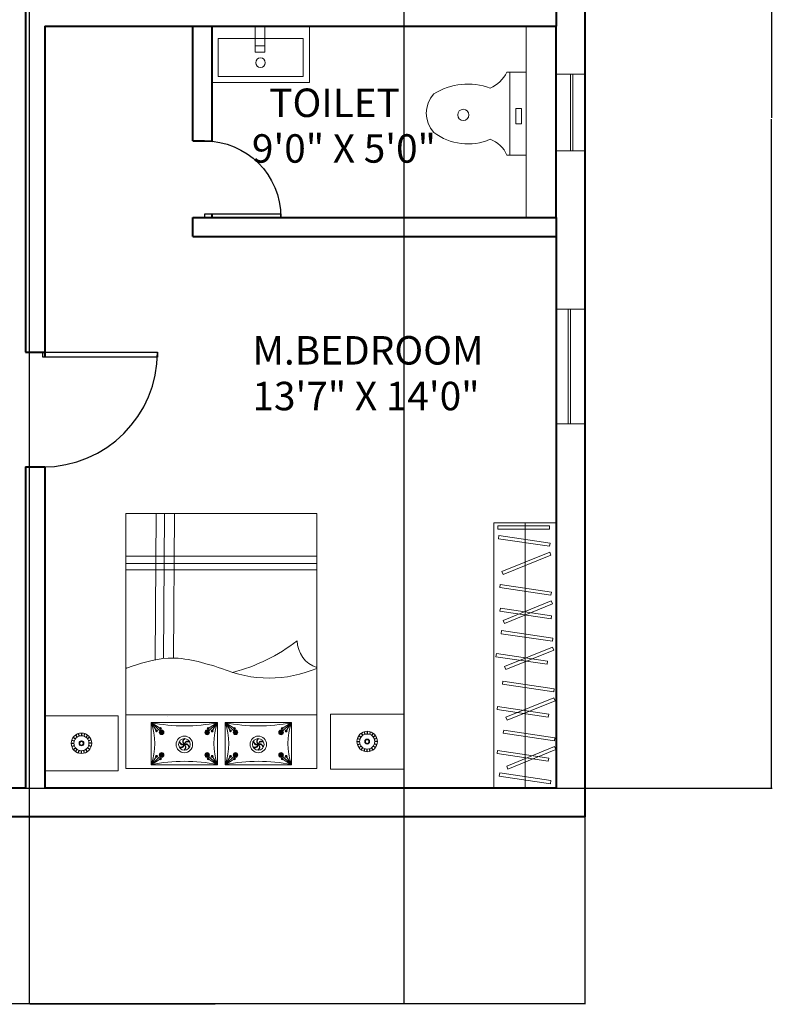
# Model space of a CAD drawing. Units: inches. Extents: x -46 to 1145, y -527 to 760.
# Tile 19 of 57: x 909 to 1145, y -527 to -218. Entities that reach past the tile are written whole.
import ezdxf

# ---------------------------------------------------------------- set-up
doc = ezdxf.new("R2010")
doc.units = ezdxf.units.IN
doc.header["$MEASUREMENT"] = 0
for name, color, linetype, lineweight in [('A-ANNO-DIMS', 2, 'Continuous', 18), ('A-AREA-IDEN', 1, 'Continuous', 18), ('A-FLOR-CASE', 32, 'Continuous', 18), ('A-FLOR-FIXT', 9, 'Continuous', 18), ('A-FURN', 2, 'Continuous', 13), ('C-SITE', 7, 'Continuous', 30), ('DOORS', 3, 'Continuous', 25), ('WALLS', 4, 'Continuous', 40), ('WINDOWS', 240, 'Continuous', 20)]:
    doc.layers.add(name, color=color, linetype=linetype, lineweight=lineweight)
doc.layers.add('FURNTIURE', color=2, linetype='Continuous')
doc.layers.add('LT', color=9, linetype='Continuous')
doc.styles.get("Standard").update_dxf_attribs({"font": 'arial.ttf'})
doc.dimstyles.get("Standard").update_dxf_attribs({"dimtxt": 0.18, "dimasz": 0.18, "dimexe": 0.18, "dimexo": 0.0625, "dimgap": 0.09, "dimtad": 0, "dimtih": 1, "dimtoh": 1, "dimdec": 0, "dimzin": 0, "dimdsep": 46, "dimlunit": 3, "dimtxsty": 'Standard', "dimcen": 0.09, "dimadec": 0, "dimazin": 0, "dimtfac": 1, "dimtdec": 0, "dimtofl": 0, "dimtmove": 0, "dimatfit": 3, "dimfxl": 1, "dimtolj": 1, "dimtzin": 0, "dimarcsym": 0})

# ---------------------------------------------------------------- blocks, each defined once
blk = doc.blocks.new('*U2')
for p, q in [((0, 0), (0, -6)), ((40, 0), (40, -6))]:
    blk.add_line(p, q)
blk.add_lwpolyline([(0, 0), (0, 40), (1.75, 40), (1.75, 0)], close=True)
blk.add_arc((0, 0), 40, 0, 90)
blk = doc.blocks.new('*U89')
at = {"layer": 'FURNTIURE'}
blk.add_line((0, 0.42), (0, -0.42), dxfattribs=at)
blk = doc.blocks.new('*U90')
at = {"layer": 'FURNTIURE', "transparency": 16777216}
for p, rotation in [((589.5, 506.39), 54), ((590.11, 507), 36), ((590.89, 507.4), 17.99999999999997), ((592.61, 507.4), 341.9999999999999), ((593.39, 507), 324), ((594.01, 506.39), 306), ((588.97, 504.75), 90), ((589.1, 505.61), 72), ((589.1, 503.89), 108), ((589.5, 503.11), 126), ((594.01, 503.11), 234), ((594.4, 505.61), 288), ((594.4, 503.89), 252), ((594.54, 504.75), 270), ((590.11, 502.49), 144), ((590.89, 502.1), 162), ((591.75, 501.96), 180), ((592.61, 502.1), 197.9999999999999), ((593.39, 502.49), 216)]:
    blk.add_blockref('*U89', p, dxfattribs=dict(at, rotation=rotation))
blk.add_blockref('*U89', (591.75, 507.53), dxfattribs=at)
blk = doc.blocks.new('*U87')
at = {"layer": 'FURNTIURE'}
blk.add_line((0, 0.1), (0, -0.1), dxfattribs=at)
blk = doc.blocks.new('*U88')
at = {"layer": 'FURNTIURE', "transparency": 16777216}
for p, rotation in [((141.23, 121.04), 90), ((141.27, 121.25), 72), ((141.27, 120.83), 108), ((141.36, 121.43), 54), ((141.36, 120.65), 126), ((141.51, 121.58), 35.99999999999999), ((141.51, 120.5), 144), ((141.7, 121.67), 17.99999999999998), ((141.7, 120.4), 162), ((141.9, 120.37), 180), ((142.11, 121.67), 342), ((142.11, 120.4), 198), ((142.3, 121.58), 324), ((142.3, 120.5), 216), ((142.44, 121.43), 306), ((142.44, 120.65), 234), ((142.54, 121.25), 288), ((142.54, 120.83), 252), ((142.57, 121.04), 270)]:
    blk.add_blockref('*U87', p, dxfattribs=dict(at, rotation=rotation))
blk.add_blockref('*U87', (141.9, 121.71), dxfattribs=at)
blk = doc.blocks.new('NIGHTSTAND')
blk.add_lwpolyline([(23.06, 0), (0, 0), (0, 17.28), (23.06, 17.28)], close=True)
for radius in [3.21, 2.36, 0.77, 0.567]:
    blk.add_circle((11.53, 8.64), radius)
for name, p in [('*U90', (-580.22, -496.1)), ('*U88', (-130.37, -112.4))]:
    blk.add_blockref(name, p)
blk = doc.blocks.new('WARDROBE')
blk.add_line((9.78, 0), (9.78, 83.25))
for points in [[(19.56, 0), (0, 0), (0, 83.25), (19.56, 83.25)], [(17.74, 78.49), (1.66, 80.88), (1.8, 81.87), (17.88, 79.48)], [(15.55, 76.35), (0.49, 70.23), (0.11, 71.16), (15.17, 77.28)], [(18.43, 71.4), (2.35, 73.79), (2.5, 74.78), (18.58, 72.39)], [(16.47, 65.03), (0.39, 67.42), (0.54, 68.41), (16.62, 66.02)], [(15.79, 61), (0.73, 54.88), (0.35, 55.81), (15.41, 61.93)], [(18.43, 57.62), (2.35, 60.01), (2.5, 61), (18.58, 58.61)], [(16.71, 49.68), (0.63, 52.07), (0.78, 53.06), (16.86, 50.67)], [(16.22, 45.12), (1.16, 39), (0.78, 39.93), (15.84, 46.05)], [(18.77, 41.02), (2.69, 43.41), (2.84, 44.4), (18.92, 42.01)], [(17.14, 33.8), (1.06, 36.19), (1.21, 37.19), (17.29, 34.8)], [(16.65, 30.67), (1.59, 24.55), (1.21, 25.48), (16.27, 31.6)], [(17.52, 26.78), (1.44, 29.17), (1.59, 30.16), (17.67, 27.77)], [(17.57, 19.35), (1.49, 21.74), (1.64, 22.73), (17.72, 20.34)], [(17.08, 15.35), (2.02, 9.23), (1.64, 10.16), (16.7, 16.28)], [(18, 4.03), (1.92, 6.42), (2.07, 7.41), (18.15, 5.03)], [(18.32, 0.98), (2.07, 0.98), (2.07, 1.98), (18.32, 1.98)]]:
    blk.add_lwpolyline(points, close=True)
blk = doc.blocks.new('LAVATORY-RECT')
blk.add_line((14.01, 6.17), (17.08, 6.17))
for points in [[(30.61, 0), (0, 0), (0, 17.7), (30.61, 17.7)], [(28.7, 3.94), (1.97, 3.94), (1.97, 15.81), (28.7, 15.81)], [(17.08, 0), (14.01, 0), (14.01, 8.17), (17.08, 8.17)]]:
    blk.add_lwpolyline(points, close=True)
blk.add_circle((15.39, 11.51), 1.51)
blk = doc.blocks.new('WATER-CLOSET')
for p, q in [((0, 0), (0, 26.01)), ((0, 26.01), (6.13, 26.01)), ((5.22, 21.04), (5.22, 26.01)), ((5.22, 26.01), (5.22, 0)), ((0, 0), (6.13, 0))]:
    blk.add_line(p, q)
blk.add_lwpolyline([(1.51, 11.4), (1.51, 16.16), (3.34, 16.16), (3.34, 11.4)], close=True)
blk.add_circle((19.79, 13.37), 1.75)
for centre, radius, start, end in [((14.15, 29.2), 8.64, 201.6782, 251.0259), ((18.35, 4.96), 17.54, 52.4616, 113.5359), ((22.52, 12.84), 8.87, 317.2682, 42.7318), ((18.33, 23.71), 20, 249.5645, 302.3709), ((15.4, -4.5), 10.31, 113.1704, 154.0947)]:
    blk.add_arc(centre, radius, start, end)
blk = doc.blocks.new('WINDOW-36IN')
for p, q in [((0, 4.5), (0, 9)), ((0, 9), (0, 0)), ((36, 9), (36, 0)), ((0, 5.23), (36, 5.23)), ((0, 4.5), (36, 4.5))]:
    blk.add_line(p, q)
blk = doc.blocks.new('WINDOW-24IN')
for p, q in [((0, 4.5), (0, 9)), ((0, 9), (0, 0)), ((24, 9), (24, 0)), ((0, 5.23), (24, 5.23)), ((0, 4.5), (24, 4.5))]:
    blk.add_line(p, q)
blk = doc.blocks.new('*U58')
at = {"layer": 'LT'}
blk.add_line((0, 0.28), (0, -0.28), dxfattribs=at)
for centre, start, end in [((0.73, 0), 159.0676, 200.9324), ((-0.73, 0), 339.0676, 20.9324)]:
    blk.add_arc(centre, 0.786, start, end, dxfattribs=at)
blk = doc.blocks.new('*U59')
at = {"layer": 'LT', "transparency": 16777216}
for p, rotation in [((609.66, 443.79), 80.00000000000001), ((609.69, 443.6), 120), ((609.76, 443.96), 40.00000000000002), ((609.84, 443.48), 160), ((610.03, 443.48), 200), ((610.12, 443.96), 320), ((610.18, 443.6), 240), ((610.21, 443.79), 280)]:
    blk.add_blockref('*U58', p, dxfattribs=dict(at, rotation=rotation))
blk.add_blockref('*U58', (609.94, 444.03), dxfattribs=at)
blk = doc.blocks.new('*U60')
at = {"layer": 'LT'}
blk.add_line((0, 0.12), (0, -0.12), dxfattribs=at)
for centre, start, end in [((0.31, 0), 159.0676, 200.9324), ((-0.31, 0), 339.0676, 20.9324)]:
    blk.add_arc(centre, 0.335, start, end, dxfattribs=at)
blk = doc.blocks.new('*U61')
at = {"layer": 'LT', "transparency": 16777216}
for p, rotation in [((259.5, 188.9), 80.00000000000001), ((259.51, 188.82), 120), ((259.54, 188.97), 40), ((259.57, 188.76), 160), ((259.65, 188.76), 200), ((259.69, 188.97), 320), ((259.72, 188.82), 240), ((259.73, 188.9), 280)]:
    blk.add_blockref('*U60', p, dxfattribs=dict(at, rotation=rotation))
blk.add_blockref('*U60', (259.61, 189), dxfattribs=at)
blk = doc.blocks.new('*U62')
at = {"layer": 'LT'}
blk.add_line((0, 0.12), (0, -0.12), dxfattribs=at)
for centre, start, end in [((0.31, 0), 159.0676, 200.9324), ((-0.31, 0), 339.0676, 20.9324)]:
    blk.add_arc(centre, 0.335, start, end, dxfattribs=at)
blk = doc.blocks.new('*U63')
at = {"layer": 'LT', "transparency": 16777216}
for p, rotation in [((259.5, 188.9), 80.00000000000001), ((259.51, 188.82), 120), ((259.54, 188.97), 40), ((259.57, 188.76), 160), ((259.65, 188.76), 200), ((259.69, 188.97), 320), ((259.72, 188.82), 240), ((259.73, 188.9), 280)]:
    blk.add_blockref('*U62', p, dxfattribs=dict(at, rotation=rotation))
blk.add_blockref('*U62', (259.61, 189), dxfattribs=at)
blk = doc.blocks.new('*U64')
at = {"layer": 'LT'}
blk.add_line((0, 0.28), (0, -0.28), dxfattribs=at)
for centre, start, end in [((0.73, 0), 159.0676, 200.9324), ((-0.73, 0), 339.0676, 20.9324)]:
    blk.add_arc(centre, 0.786, start, end, dxfattribs=at)
blk = doc.blocks.new('*U65')
at = {"layer": 'LT', "transparency": 16777216}
for p, rotation in [((609.66, 443.79), 80.00000000000001), ((609.69, 443.6), 120), ((609.76, 443.96), 40.00000000000002), ((609.84, 443.48), 160), ((610.03, 443.48), 200), ((610.12, 443.96), 320), ((610.18, 443.6), 240), ((610.21, 443.79), 280)]:
    blk.add_blockref('*U64', p, dxfattribs=dict(at, rotation=rotation))
blk.add_blockref('*U64', (609.94, 444.03), dxfattribs=at)
blk = doc.blocks.new('*U66')
at = {"layer": 'LT'}
blk.add_line((0, 0.12), (0, -0.12), dxfattribs=at)
for centre, start, end in [((0.31, 0), 159.0676, 200.9324), ((-0.31, 0), 339.0676, 20.9324)]:
    blk.add_arc(centre, 0.335, start, end, dxfattribs=at)
blk = doc.blocks.new('*U67')
at = {"layer": 'LT', "transparency": 16777216}
for p, rotation in [((259.5, 188.9), 80.00000000000001), ((259.51, 188.82), 120), ((259.54, 188.97), 40), ((259.57, 188.76), 160), ((259.65, 188.76), 200), ((259.69, 188.97), 320), ((259.72, 188.82), 240), ((259.73, 188.9), 280)]:
    blk.add_blockref('*U66', p, dxfattribs=dict(at, rotation=rotation))
blk.add_blockref('*U66', (259.61, 189), dxfattribs=at)
blk = doc.blocks.new('*U68')
at = {"layer": 'LT'}
blk.add_line((0, 0.12), (0, -0.12), dxfattribs=at)
for centre, start, end in [((0.31, 0), 159.0676, 200.9324), ((-0.31, 0), 339.0676, 20.9324)]:
    blk.add_arc(centre, 0.335, start, end, dxfattribs=at)
blk = doc.blocks.new('*U69')
at = {"layer": 'LT', "transparency": 16777216}
for p, rotation in [((259.5, 188.9), 80.00000000000001), ((259.51, 188.82), 120), ((259.54, 188.97), 40), ((259.57, 188.76), 160), ((259.65, 188.76), 200), ((259.69, 188.97), 320), ((259.72, 188.82), 240), ((259.73, 188.9), 280)]:
    blk.add_blockref('*U68', p, dxfattribs=dict(at, rotation=rotation))
blk.add_blockref('*U68', (259.61, 189), dxfattribs=at)
blk = doc.blocks.new('*U70')
at = {"layer": 'LT'}
blk.add_line((0, 0.28), (0, -0.28), dxfattribs=at)
for centre, start, end in [((0.73, 0), 159.0676, 200.9324), ((-0.73, 0), 339.0676, 20.9324)]:
    blk.add_arc(centre, 0.786, start, end, dxfattribs=at)
blk = doc.blocks.new('*U71')
at = {"layer": 'LT', "transparency": 16777216}
for p, rotation in [((609.66, 443.79), 80.00000000000001), ((609.69, 443.6), 120), ((609.76, 443.96), 40.00000000000002), ((609.84, 443.48), 160), ((610.03, 443.48), 200), ((610.12, 443.96), 320), ((610.18, 443.6), 240), ((610.21, 443.79), 280)]:
    blk.add_blockref('*U70', p, dxfattribs=dict(at, rotation=rotation))
blk.add_blockref('*U70', (609.94, 444.03), dxfattribs=at)
blk = doc.blocks.new('*U46')
at = {"layer": 'LT'}
blk.add_line((0, 0.12), (0, -0.12), dxfattribs=at)
for centre, start, end in [((0.31, 0), 159.0676, 200.9324), ((-0.31, 0), 339.0676, 20.9324)]:
    blk.add_arc(centre, 0.335, start, end, dxfattribs=at)
blk = doc.blocks.new('*U47')
at = {"layer": 'LT', "transparency": 16777216}
for p, rotation in [((259.5, 188.9), 80.00000000000001), ((259.51, 188.82), 120), ((259.54, 188.97), 40), ((259.57, 188.76), 160), ((259.65, 188.76), 200), ((259.69, 188.97), 320), ((259.72, 188.82), 240), ((259.73, 188.9), 280)]:
    blk.add_blockref('*U46', p, dxfattribs=dict(at, rotation=rotation))
blk.add_blockref('*U46', (259.61, 189), dxfattribs=at)
blk = doc.blocks.new('*U48')
at = {"layer": 'LT'}
blk.add_line((0, 0.12), (0, -0.12), dxfattribs=at)
for centre, start, end in [((0.31, 0), 159.0676, 200.9324), ((-0.31, 0), 339.0676, 20.9324)]:
    blk.add_arc(centre, 0.335, start, end, dxfattribs=at)
blk = doc.blocks.new('*U49')
at = {"layer": 'LT', "transparency": 16777216}
for p, rotation in [((259.5, 188.9), 80.00000000000001), ((259.51, 188.82), 120), ((259.54, 188.97), 40), ((259.57, 188.76), 160), ((259.65, 188.76), 200), ((259.69, 188.97), 320), ((259.72, 188.82), 240), ((259.73, 188.9), 280)]:
    blk.add_blockref('*U48', p, dxfattribs=dict(at, rotation=rotation))
blk.add_blockref('*U48', (259.61, 189), dxfattribs=at)
blk = doc.blocks.new('*U50')
at = {"layer": 'LT'}
blk.add_line((0, 0.28), (0, -0.28), dxfattribs=at)
for centre, start, end in [((0.73, 0), 159.0676, 200.9324), ((-0.73, 0), 339.0676, 20.9324)]:
    blk.add_arc(centre, 0.786, start, end, dxfattribs=at)
blk = doc.blocks.new('*U51')
at = {"layer": 'LT', "transparency": 16777216}
for p, rotation in [((609.66, 443.79), 80.00000000000001), ((609.69, 443.6), 120), ((609.76, 443.96), 40.00000000000002), ((609.84, 443.48), 160), ((610.03, 443.48), 200), ((610.12, 443.96), 320), ((610.18, 443.6), 240), ((610.21, 443.79), 280)]:
    blk.add_blockref('*U50', p, dxfattribs=dict(at, rotation=rotation))
blk.add_blockref('*U50', (609.94, 444.03), dxfattribs=at)
blk = doc.blocks.new('*U52')
at = {"layer": 'LT'}
blk.add_line((0, 0.12), (0, -0.12), dxfattribs=at)
for centre, start, end in [((0.31, 0), 159.0676, 200.9324), ((-0.31, 0), 339.0676, 20.9324)]:
    blk.add_arc(centre, 0.335, start, end, dxfattribs=at)
blk = doc.blocks.new('*U53')
at = {"layer": 'LT', "transparency": 16777216}
for p, rotation in [((259.5, 188.9), 80.00000000000001), ((259.51, 188.82), 120), ((259.54, 188.97), 40), ((259.57, 188.76), 160), ((259.65, 188.76), 200), ((259.69, 188.97), 320), ((259.72, 188.82), 240), ((259.73, 188.9), 280)]:
    blk.add_blockref('*U52', p, dxfattribs=dict(at, rotation=rotation))
blk.add_blockref('*U52', (259.61, 189), dxfattribs=at)
blk = doc.blocks.new('*U54')
at = {"layer": 'LT'}
blk.add_line((0, 0.12), (0, -0.12), dxfattribs=at)
for centre, start, end in [((0.31, 0), 159.0676, 200.9324), ((-0.31, 0), 339.0676, 20.9324)]:
    blk.add_arc(centre, 0.335, start, end, dxfattribs=at)
blk = doc.blocks.new('*U55')
at = {"layer": 'LT', "transparency": 16777216}
for p, rotation in [((259.5, 188.9), 80.00000000000001), ((259.51, 188.82), 120), ((259.54, 188.97), 40), ((259.57, 188.76), 160), ((259.65, 188.76), 200), ((259.69, 188.97), 320), ((259.72, 188.82), 240), ((259.73, 188.9), 280)]:
    blk.add_blockref('*U54', p, dxfattribs=dict(at, rotation=rotation))
blk.add_blockref('*U54', (259.61, 189), dxfattribs=at)
blk = doc.blocks.new('*U34')
at = {"layer": 'LT'}
blk.add_line((0, 0.28), (0, -0.28), dxfattribs=at)
for centre, start, end in [((0.73, 0), 159.0676, 200.9324), ((-0.73, 0), 339.0676, 20.9324)]:
    blk.add_arc(centre, 0.786, start, end, dxfattribs=at)
blk = doc.blocks.new('*U35')
at = {"layer": 'LT', "transparency": 16777216}
for p, rotation in [((609.66, 443.79), 80.00000000000001), ((609.69, 443.6), 120), ((609.76, 443.96), 40.00000000000002), ((609.84, 443.48), 160), ((610.03, 443.48), 200), ((610.12, 443.96), 320), ((610.18, 443.6), 240), ((610.21, 443.79), 280)]:
    blk.add_blockref('*U34', p, dxfattribs=dict(at, rotation=rotation))
blk.add_blockref('*U34', (609.94, 444.03), dxfattribs=at)
blk = doc.blocks.new('*U36')
at = {"layer": 'LT'}
blk.add_line((0, 0.12), (0, -0.12), dxfattribs=at)
for centre, start, end in [((0.31, 0), 159.0676, 200.9324), ((-0.31, 0), 339.0676, 20.9324)]:
    blk.add_arc(centre, 0.335, start, end, dxfattribs=at)
blk = doc.blocks.new('*U37')
at = {"layer": 'LT', "transparency": 16777216}
for p, rotation in [((259.5, 188.9), 80.00000000000001), ((259.51, 188.82), 120), ((259.54, 188.97), 40), ((259.57, 188.76), 160), ((259.65, 188.76), 200), ((259.69, 188.97), 320), ((259.72, 188.82), 240), ((259.73, 188.9), 280)]:
    blk.add_blockref('*U36', p, dxfattribs=dict(at, rotation=rotation))
blk.add_blockref('*U36', (259.61, 189), dxfattribs=at)
blk = doc.blocks.new('*U38')
at = {"layer": 'LT'}
blk.add_line((0, 0.12), (0, -0.12), dxfattribs=at)
for centre, start, end in [((0.31, 0), 159.0676, 200.9324), ((-0.31, 0), 339.0676, 20.9324)]:
    blk.add_arc(centre, 0.335, start, end, dxfattribs=at)
blk = doc.blocks.new('*U39')
at = {"layer": 'LT', "transparency": 16777216}
for p, rotation in [((259.5, 188.9), 80.00000000000001), ((259.51, 188.82), 120), ((259.54, 188.97), 40), ((259.57, 188.76), 160), ((259.65, 188.76), 200), ((259.69, 188.97), 320), ((259.72, 188.82), 240), ((259.73, 188.9), 280)]:
    blk.add_blockref('*U38', p, dxfattribs=dict(at, rotation=rotation))
blk.add_blockref('*U38', (259.61, 189), dxfattribs=at)
blk = doc.blocks.new('*U40')
at = {"layer": 'LT'}
blk.add_line((0, 0.28), (0, -0.28), dxfattribs=at)
for centre, start, end in [((0.73, 0), 159.0676, 200.9324), ((-0.73, 0), 339.0676, 20.9324)]:
    blk.add_arc(centre, 0.786, start, end, dxfattribs=at)
blk = doc.blocks.new('*U41')
at = {"layer": 'LT', "transparency": 16777216}
for p, rotation in [((609.66, 443.79), 80.00000000000001), ((609.69, 443.6), 120), ((609.76, 443.96), 40.00000000000002), ((609.84, 443.48), 160), ((610.03, 443.48), 200), ((610.12, 443.96), 320), ((610.18, 443.6), 240), ((610.21, 443.79), 280)]:
    blk.add_blockref('*U40', p, dxfattribs=dict(at, rotation=rotation))
blk.add_blockref('*U40', (609.94, 444.03), dxfattribs=at)
blk = doc.blocks.new('*U42')
at = {"layer": 'LT'}
blk.add_line((0, 0.12), (0, -0.12), dxfattribs=at)
for centre, start, end in [((0.31, 0), 159.0676, 200.9324), ((-0.31, 0), 339.0676, 20.9324)]:
    blk.add_arc(centre, 0.335, start, end, dxfattribs=at)
blk = doc.blocks.new('*U43')
at = {"layer": 'LT', "transparency": 16777216}
for p, rotation in [((259.5, 188.9), 80.00000000000001), ((259.51, 188.82), 120), ((259.54, 188.97), 40), ((259.57, 188.76), 160), ((259.65, 188.76), 200), ((259.69, 188.97), 320), ((259.72, 188.82), 240), ((259.73, 188.9), 280)]:
    blk.add_blockref('*U42', p, dxfattribs=dict(at, rotation=rotation))
blk.add_blockref('*U42', (259.61, 189), dxfattribs=at)
blk = doc.blocks.new('*U44')
at = {"layer": 'LT'}
blk.add_line((0, 0.12), (0, -0.12), dxfattribs=at)
for centre, start, end in [((0.31, 0), 159.0676, 200.9324), ((-0.31, 0), 339.0676, 20.9324)]:
    blk.add_arc(centre, 0.335, start, end, dxfattribs=at)
blk = doc.blocks.new('*U45')
at = {"layer": 'LT', "transparency": 16777216}
for p, rotation in [((259.5, 188.9), 80.00000000000001), ((259.51, 188.82), 120), ((259.54, 188.97), 40), ((259.57, 188.76), 160), ((259.65, 188.76), 200), ((259.69, 188.97), 320), ((259.72, 188.82), 240), ((259.73, 188.9), 280)]:
    blk.add_blockref('*U44', p, dxfattribs=dict(at, rotation=rotation))
blk.add_blockref('*U44', (259.61, 189), dxfattribs=at)
blk = doc.blocks.new('*U72')
at = {"layer": 'LT'}
blk.add_line((0, 0.28), (0, -0.28), dxfattribs=at)
for centre, start, end in [((0.73, 0), 159.0676, 200.9324), ((-0.73, 0), 339.0676, 20.9324)]:
    blk.add_arc(centre, 0.786, start, end, dxfattribs=at)
blk = doc.blocks.new('*U73')
at = {"layer": 'LT', "transparency": 16777216}
for p, rotation in [((609.66, 443.79), 80.00000000000001), ((609.69, 443.6), 120), ((609.76, 443.96), 40.00000000000002), ((609.84, 443.48), 160), ((610.03, 443.48), 200), ((610.12, 443.96), 320), ((610.18, 443.6), 240), ((610.21, 443.79), 280)]:
    blk.add_blockref('*U72', p, dxfattribs=dict(at, rotation=rotation))
blk.add_blockref('*U72', (609.94, 444.03), dxfattribs=at)
blk = doc.blocks.new('*U74')
at = {"layer": 'LT'}
blk.add_line((0, 0.12), (0, -0.12), dxfattribs=at)
for centre, start, end in [((0.31, 0), 159.0676, 200.9324), ((-0.31, 0), 339.0676, 20.9324)]:
    blk.add_arc(centre, 0.335, start, end, dxfattribs=at)
blk = doc.blocks.new('*U75')
at = {"layer": 'LT', "transparency": 16777216}
for p, rotation in [((259.5, 188.9), 80.00000000000001), ((259.51, 188.82), 120), ((259.54, 188.97), 40), ((259.57, 188.76), 160), ((259.65, 188.76), 200), ((259.69, 188.97), 320), ((259.72, 188.82), 240), ((259.73, 188.9), 280)]:
    blk.add_blockref('*U74', p, dxfattribs=dict(at, rotation=rotation))
blk.add_blockref('*U74', (259.61, 189), dxfattribs=at)
blk = doc.blocks.new('*U76')
at = {"layer": 'LT'}
blk.add_line((0, 0.12), (0, -0.12), dxfattribs=at)
for centre, start, end in [((0.31, 0), 159.0676, 200.9324), ((-0.31, 0), 339.0676, 20.9324)]:
    blk.add_arc(centre, 0.335, start, end, dxfattribs=at)
blk = doc.blocks.new('*U77')
at = {"layer": 'LT', "transparency": 16777216}
for p, rotation in [((259.5, 188.9), 80.00000000000001), ((259.51, 188.82), 120), ((259.54, 188.97), 40), ((259.57, 188.76), 160), ((259.65, 188.76), 200), ((259.69, 188.97), 320), ((259.72, 188.82), 240), ((259.73, 188.9), 280)]:
    blk.add_blockref('*U76', p, dxfattribs=dict(at, rotation=rotation))
blk.add_blockref('*U76', (259.61, 189), dxfattribs=at)
blk = doc.blocks.new('*U78')
at = {"layer": 'LT'}
blk.add_line((0, 0.28), (0, -0.28), dxfattribs=at)
for centre, start, end in [((0.73, 0), 159.0676, 200.9324), ((-0.73, 0), 339.0676, 20.9324)]:
    blk.add_arc(centre, 0.786, start, end, dxfattribs=at)
blk = doc.blocks.new('*U79')
at = {"layer": 'LT', "transparency": 16777216}
for p, rotation in [((609.66, 443.79), 80.00000000000001), ((609.69, 443.6), 120), ((609.76, 443.96), 40.00000000000002), ((609.84, 443.48), 160), ((610.03, 443.48), 200), ((610.12, 443.96), 320), ((610.18, 443.6), 240), ((610.21, 443.79), 280)]:
    blk.add_blockref('*U78', p, dxfattribs=dict(at, rotation=rotation))
blk.add_blockref('*U78', (609.94, 444.03), dxfattribs=at)
blk = doc.blocks.new('*U80')
at = {"layer": 'LT'}
blk.add_line((0, 0.12), (0, -0.12), dxfattribs=at)
for centre, start, end in [((0.31, 0), 159.0676, 200.9324), ((-0.31, 0), 339.0676, 20.9324)]:
    blk.add_arc(centre, 0.335, start, end, dxfattribs=at)
blk = doc.blocks.new('*U81')
at = {"layer": 'LT', "transparency": 16777216}
for p, rotation in [((259.5, 188.9), 80.00000000000001), ((259.51, 188.82), 120), ((259.54, 188.97), 40), ((259.57, 188.76), 160), ((259.65, 188.76), 200), ((259.69, 188.97), 320), ((259.72, 188.82), 240), ((259.73, 188.9), 280)]:
    blk.add_blockref('*U80', p, dxfattribs=dict(at, rotation=rotation))
blk.add_blockref('*U80', (259.61, 189), dxfattribs=at)
blk = doc.blocks.new('*U82')
at = {"layer": 'LT'}
blk.add_line((0, 0.12), (0, -0.12), dxfattribs=at)
for centre, start, end in [((0.31, 0), 159.0676, 200.9324), ((-0.31, 0), 339.0676, 20.9324)]:
    blk.add_arc(centre, 0.335, start, end, dxfattribs=at)
blk = doc.blocks.new('*U83')
at = {"layer": 'LT', "transparency": 16777216}
for p, rotation in [((259.5, 188.9), 80.00000000000001), ((259.51, 188.82), 120), ((259.54, 188.97), 40), ((259.57, 188.76), 160), ((259.65, 188.76), 200), ((259.69, 188.97), 320), ((259.72, 188.82), 240), ((259.73, 188.9), 280)]:
    blk.add_blockref('*U82', p, dxfattribs=dict(at, rotation=rotation))
blk.add_blockref('*U82', (259.61, 189), dxfattribs=at)
blk = doc.blocks.new('*U32')
at = {"layer": 'FURNTIURE'}
blk.add_open_spline([(0.04, 1.82), (-0.22, 1.45), (-0.66, 0.8), (0.1, -0.02), (0.64, -0.93), (0.24, -1.53), (0.04, -1.82)], degree=3, knots=[0, 0, 0, 0, 1.177175, 2.037162, 3.056205, 4.032246, 4.032246, 4.032246, 4.032246], dxfattribs=at)
blk = doc.blocks.new('*U33')
at = {"layer": 'FURNTIURE', "transparency": 16777216}
for p, rotation in [((904.32, 663.42), 300), ((904.32, 663.35), 59.99999999999999), ((904.36, 663.42), 239.9999999999999), ((904.36, 663.35), 119.9999999999999), ((904.38, 663.38), 180)]:
    blk.add_blockref('*U32', p, dxfattribs=dict(at, rotation=rotation))
blk.add_blockref('*U32', (904.3, 663.38), dxfattribs=at)
blk = doc.blocks.new('*U56')
at = {"layer": 'FURNTIURE'}
blk.add_open_spline([(0.04, 1.82), (-0.22, 1.45), (-0.66, 0.8), (0.1, -0.02), (0.64, -0.93), (0.24, -1.53), (0.04, -1.82)], degree=3, knots=[0, 0, 0, 0, 1.177175, 2.037162, 3.056205, 4.032246, 4.032246, 4.032246, 4.032246], dxfattribs=at)
blk = doc.blocks.new('*U57')
at = {"layer": 'FURNTIURE', "transparency": 16777216}
for p, rotation in [((904.32, 663.42), 300), ((904.32, 663.35), 59.99999999999999), ((904.36, 663.42), 239.9999999999999), ((904.36, 663.35), 119.9999999999999), ((904.38, 663.38), 180)]:
    blk.add_blockref('*U56', p, dxfattribs=dict(at, rotation=rotation))
blk.add_blockref('*U56', (904.3, 663.38), dxfattribs=at)
blk = doc.blocks.new('BED-QUEEN-FURNISHED')
for p, q in [((0, 0), (0, 80)), ((0, 80), (60, 80)), ((8, 78.8), (28.8, 78.8)), ((8, 65.6), (8, 78.8)), ((8, 78.8), (11.38, 75.61)), ((8, 78.8), (9.68, 76.18)), ((8, 78.8), (10.93, 76.98)), ((28.8, 78.8), (25.41, 75.61)), ((28.8, 78.8), (25.87, 76.98)), ((28.8, 78.8), (27.12, 76.18)), ((28.8, 78.8), (28.8, 65.6)), ((31.2, 78.8), (52, 78.8)), ((31.2, 65.6), (31.2, 78.8)), ((31.2, 78.8), (52, 78.8)), ((31.2, 65.6), (31.2, 78.8)), ((31.2, 78.8), (34.58, 75.61)), ((31.2, 78.8), (32.88, 76.18)), ((31.2, 78.8), (34.13, 76.98)), ((52, 78.8), (48.61, 75.61)), ((52, 78.8), (49.07, 76.98)), ((52, 78.8), (50.32, 76.18)), ((52, 78.8), (52, 65.6)), ((52, 78.8), (52, 65.6)), ((60, 80), (60, 0)), ((10.93, 76.98), (10.93, 76.75)), ((11.25, 75.74), (11.25, 75.18)), ((25.55, 75.74), (25.55, 75.18)), ((25.87, 76.98), (25.87, 76.75)), ((27.12, 76.18), (27.12, 75.95)), ((34.13, 76.98), (34.13, 76.75)), ((34.45, 75.74), (34.45, 75.18)), ((48.75, 75.74), (48.75, 75.18)), ((49.07, 76.98), (49.07, 76.75)), ((50.32, 76.18), (50.32, 75.95)), ((8, 65.61), (11.38, 68.8)), ((8, 65.61), (9.68, 68.23)), ((11.25, 68.67), (11.25, 69.23)), ((28.8, 65.6), (25.41, 68.79)), ((27.11, 68.22), (27.11, 68.46)), ((28.8, 65.6), (27.11, 68.22)), ((31.2, 65.61), (34.58, 68.8)), ((31.2, 65.61), (32.88, 68.23)), ((34.45, 68.67), (34.45, 69.23)), ((52, 65.6), (48.61, 68.79)), ((50.31, 68.22), (50.31, 68.46)), ((52, 65.6), (50.31, 68.22)), ((8, 65.61), (10.92, 67.43)), ((8, 65.6), (28.8, 65.6)), ((10.92, 67.43), (10.92, 67.67)), ((25.87, 67.42), (25.87, 67.66)), ((28.8, 65.6), (25.87, 67.42)), ((31.2, 65.61), (34.12, 67.43)), ((31.2, 65.6), (52, 65.6)), ((31.2, 65.6), (52, 65.6)), ((34.12, 67.43), (34.12, 67.67)), ((49.07, 67.42), (49.07, 67.66)), ((52, 65.6), (49.07, 67.42)), ((60, 63.2), (0, 63.2)), ((46.8, 63.6), (46.8, 63.6)), ((44.72, 0), (45.02, 45.37)), ((47.8, 0), (48.1, 45.5)), ((50.46, 0), (50.76, 45.91)), ((0, 17.7), (60, 17.7)), ((0, 15.69), (60, 15.69)), ((0, 13.42), (60, 13.42)), ((60, 0), (0, 0))]:
    blk.add_line(p, q)
for centre, radius in [((10.93, 76.98), 0.308), ((10.93, 76.98), 0.239), ((25.87, 76.98), 0.308), ((25.87, 76.98), 0.239), ((34.13, 76.98), 0.308), ((34.13, 76.98), 0.239), ((49.07, 76.98), 0.308), ((49.07, 76.98), 0.239), ((9.68, 76.18), 0.308), ((9.68, 76.18), 0.239), ((11.25, 75.74), 0.723), ((11.25, 75.74), 0.562), ((18.4, 72.44), 2.6), ((18.4, 72.44), 1.82), ((25.55, 75.74), 0.723), ((25.55, 75.74), 0.562), ((27.12, 76.18), 0.308), ((27.12, 76.18), 0.239), ((32.88, 76.18), 0.308), ((32.88, 76.18), 0.239), ((34.45, 75.74), 0.723), ((34.45, 75.74), 0.562), ((41.6, 72.44), 2.6), ((41.6, 72.44), 1.82), ((48.75, 75.74), 0.723), ((48.75, 75.74), 0.562), ((50.32, 76.18), 0.308), ((50.32, 76.18), 0.239), ((9.68, 68.23), 0.308), ((9.68, 68.23), 0.239), ((11.25, 68.67), 0.723), ((11.25, 68.67), 0.562), ((25.55, 68.66), 0.723), ((25.55, 68.66), 0.562), ((27.11, 68.22), 0.308), ((27.11, 68.22), 0.239), ((32.88, 68.23), 0.308), ((32.88, 68.23), 0.239), ((34.45, 68.67), 0.723), ((34.45, 68.67), 0.562), ((48.75, 68.66), 0.723), ((48.75, 68.66), 0.562), ((50.31, 68.22), 0.308), ((50.31, 68.22), 0.239), ((10.92, 67.43), 0.308), ((10.92, 67.43), 0.239), ((25.87, 67.42), 0.308), ((25.87, 67.42), 0.239), ((34.12, 67.43), 0.308), ((34.12, 67.43), 0.239), ((49.07, 67.42), 0.308), ((49.07, 67.42), 0.239)]:
    blk.add_circle(centre, radius)
for centre, radius, start, end in [((18.4, 129.18), 51.44, 258.3356, 281.6644), ((-10.65, 72.2), 19.79, 340.5151, 19.4849), ((47.45, 72.2), 19.79, 160.5151, 199.4849), ((41.6, 129.18), 51.44, 258.3356, 281.6644), ((12.55, 72.2), 19.79, 340.5151, 19.4849), ((70.65, 72.2), 19.79, 160.5151, 199.4849), ((11.24, 76.86), 0.335, 159.0676, 200.9324), ((10.61, 76.86), 0.335, 339.0676, 20.9324), ((11.99, 75.46), 0.786, 159.0676, 200.9324), ((10.52, 75.46), 0.786, 339.0676, 20.9324), ((26.28, 75.46), 0.786, 159.0676, 200.9324), ((24.81, 75.46), 0.786, 339.0676, 20.9324), ((26.19, 76.86), 0.335, 159.0676, 200.9324), ((25.56, 76.86), 0.335, 339.0676, 20.9324), ((27.43, 76.06), 0.335, 159.0676, 200.9324), ((26.8, 76.06), 0.335, 339.0676, 20.9324), ((34.44, 76.86), 0.335, 159.0676, 200.9324), ((33.81, 76.86), 0.335, 339.0676, 20.9324), ((35.19, 75.46), 0.786, 159.0676, 200.9324), ((33.72, 75.46), 0.786, 339.0676, 20.9324), ((49.48, 75.46), 0.786, 159.0676, 200.9324), ((48.01, 75.46), 0.786, 339.0676, 20.9324), ((49.39, 76.86), 0.335, 159.0676, 200.9324), ((48.76, 76.86), 0.335, 339.0676, 20.9324), ((50.63, 76.06), 0.335, 159.0676, 200.9324), ((50, 76.06), 0.335, 339.0676, 20.9324), ((11.98, 68.95), 0.786, 159.028, 200.8928), ((10.51, 68.95), 0.786, 339.028, 20.8928), ((27.43, 68.34), 0.335, 159.028, 200.8928), ((26.8, 68.34), 0.335, 339.028, 20.8928), ((35.18, 68.95), 0.786, 159.028, 200.8928), ((33.71, 68.95), 0.786, 339.028, 20.8928), ((50.63, 68.34), 0.335, 159.028, 200.8928), ((50, 68.34), 0.335, 339.028, 20.8928), ((18.4, 15.22), 51.44, 78.3356, 101.6644), ((11.24, 67.55), 0.335, 159.028, 200.8928), ((10.61, 67.55), 0.335, 339.028, 20.8928), ((26.18, 67.54), 0.335, 159.028, 200.8928), ((25.56, 67.54), 0.335, 339.028, 20.8928), ((41.6, 15.22), 51.44, 78.3356, 101.6644), ((34.44, 67.55), 0.335, 159.028, 200.8928), ((33.81, 67.55), 0.335, 339.028, 20.8928), ((49.38, 67.54), 0.335, 159.028, 200.8928), ((48.76, 67.54), 0.335, 339.028, 20.8928), ((15, 13.08), 38.56, 67.1089, 112.8911), ((40.88, -5.13), 56.88, 104.6834, 127.6009), ((-2.62, 39.94), 8.8, 0, 72.6522), ((40.88, -5.13), 56.88, 70.3635, 70.606)]:
    blk.add_arc(centre, radius, start, end)
blk.add_open_spline([(30, 48.6), (35.57, 46.87), (45.64, 43.74), (55.56, 47.1), (60, 48.6)], degree=3, knots=[0, 0, 0, 0, 16.971495, 30.687365, 30.687365, 30.687365, 30.687365])
at = {"xscale": -1}
for name, p in [('*U45', (270.54, -111.89)), ('*U69', (293.74, -111.89)), ('*U43', (269.3, -112.69)), ('*U41', (621.19, -368.01)), ('*U67', (292.5, -112.69)), ('*U65', (644.39, -368.01))]:
    blk.add_blockref(name, p, dxfattribs=at)
for name, p in [('*U39', (-233.74, -111.89)), ('*U63', (-210.54, -111.89)), ('*U33', (-885.94, -590.95)), ('*U35', (-584.39, -368.01)), ('*U37', (-232.5, -112.69)), ('*U57', (-862.74, -590.95)), ('*U59', (-561.19, -368.01)), ('*U61', (-209.3, -112.69))]:
    blk.add_blockref(name, p)
at = {"rotation": 179.9603994254766}
for name, p in [('*U81', (269.43, 256.92)), ('*U79', (621.49, 512)), ('*U53', (292.63, 256.92)), ('*U51', (644.69, 512)), ('*U83', (270.67, 256.12)), ('*U55', (293.87, 256.12))]:
    blk.add_blockref(name, p, dxfattribs=at)
at = {"xscale": -1, "rotation": 179.9603994254766}
for name, p in [('*U73', (-584.08, 512.83)), ('*U75', (-232.37, 257.27)), ('*U71', (-560.88, 512.83)), ('*U47', (-209.17, 257.27)), ('*U77', (-233.61, 256.47)), ('*U49', (-210.41, 256.47))]:
    blk.add_blockref(name, p, dxfattribs=at)
blk = doc.blocks.new('*D684')
at = {"layer": 'A-ANNO-DIMS', "color": 0, "lineweight": -2, "transparency": 16777216}
for p, q in [((12.56, -468.54), (12.56, -527.26)), ((1086.56, -468.54), (1086.56, -527.26)), ((12.74, -527.08), (549.21, -527.08)), ((1086.38, -527.08), (549.91, -527.08))]:
    blk.add_line(p, q, dxfattribs=at)
at = {"layer": 'A-ANNO-DIMS', "color": 0, "transparency": 16777216}
for points in [[(12.74, -527.05), (12.74, -527.11), (12.56, -527.08)], [(1086.38, -527.05), (1086.38, -527.11), (1086.56, -527.08)]]:
    blk.add_solid(points, dxfattribs=at)
at = {"layer": 'Defpoints', "color": 0, "transparency": 16777216}
for p in [(12.56, -468.48), (1086.56, -468.48), (1086.56, -527.08)]:
    blk.add_point(p, dxfattribs=at)
at = {"layer": 'A-ANNO-DIMS', "color": 0, "transparency": 16777216, "insert": (549.56, -527.08), "char_height": 0.18, "attachment_point": 5}
blk.add_mtext('\\A1;1074', dxfattribs=at)
blk = doc.blocks.new('*D694')
at = {"layer": 'A-ANNO-DIMS', "color": 0, "lineweight": -2, "transparency": 16777216}
for p, q in [((912.18, 101.46), (912.18, -527.26)), ((1029.77, 101.46), (1029.77, -527.26)), ((912.36, -527.08), (970.59, -527.08)), ((1029.59, -527.08), (971.36, -527.08))]:
    blk.add_line(p, q, dxfattribs=at)
at = {"layer": 'A-ANNO-DIMS', "color": 0, "transparency": 16777216}
for points in [[(912.36, -527.05), (912.36, -527.11), (912.18, -527.08)], [(1029.59, -527.05), (1029.59, -527.11), (1029.77, -527.08)]]:
    blk.add_solid(points, dxfattribs=at)
at = {"layer": 'Defpoints', "color": 0, "transparency": 16777216}
for p in [(912.18, 101.52), (1029.77, 101.52), (1029.77, -527.08)]:
    blk.add_point(p, dxfattribs=at)
at = {"layer": 'A-ANNO-DIMS', "color": 0, "transparency": 16777216, "insert": (970.97, -527.08), "char_height": 0.18, "attachment_point": 5}
blk.add_mtext('\\A1;117.6', dxfattribs=at)
blk = doc.blocks.new('*D702')
at = {"layer": 'A-ANNO-DIMS', "color": 0, "lineweight": -2, "transparency": 16777216}
for p, q in [((189.63, -39.48), (1145.34, -39.48)), ((1145.16, -39.66), (1145.16, -249.3)), ((1145.16, -459.3), (1145.16, -249.66)), ((183.63, -459.48), (1145.34, -459.48))]:
    blk.add_line(p, q, dxfattribs=at)
at = {"layer": 'A-ANNO-DIMS', "color": 0, "transparency": 16777216}
for points in [[(1145.13, -39.66), (1145.19, -39.66), (1145.16, -39.48)], [(1145.13, -459.3), (1145.19, -459.3), (1145.16, -459.48)]]:
    blk.add_solid(points, dxfattribs=at)
at = {"layer": 'Defpoints', "color": 0, "transparency": 16777216}
for p in [(189.56, -39.48), (1145.16, -39.48), (183.56, -459.48)]:
    blk.add_point(p, dxfattribs=at)
at = {"layer": 'A-ANNO-DIMS', "color": 0, "transparency": 16777216, "insert": (1145.16, -249.48), "char_height": 0.18, "attachment_point": 5}
blk.add_mtext('\\A1;420', dxfattribs=at)

msp = doc.modelspace()

# ---------------------------------------------------------------- linework, layer by layer
at = {"layer": 'A-FLOR-CASE'}
msp.add_line((1068.1812, -280.4824), (1068.1812, -220.4824), dxfattribs=at)
at = {"layer": 'C-SITE'}
for p, q in [((21.5637, -459.4824), (1077.5637, -459.4824)), ((12.5637, -468.4824), (1086.5637, -468.4824))]:
    msp.add_line(p, q, dxfattribs=at)
at = {"layer": 'WALLS'}
for p, q in [((1086.5637, -30.4824), (1086.5637, -468.4824)), ((911.0637, -214.4824), (911.0637, -322.768)), ((1077.5637, -214.4824), (1077.5637, -220.4824)), ((917.0637, -220.4824), (917.0637, -324.343)), ((917.0637, -220.4824), (1077.5637, -220.4824)), ((963.5637, -256.4824), (963.5637, -220.4824)), ((969.5637, -256.6027), (969.5637, -220.4824)), ((1077.5637, -280.4824), (1077.5637, -220.4824)), ((963.5637, -256.4824), (969.5637, -256.6027)), ((963.5637, -280.4824), (1077.5637, -280.4824)), ((963.5637, -286.4824), (963.5637, -280.4824)), ((963.5637, -280.4824), (969.5637, -280.4824)), ((969.5637, -280.4824), (969.5637, -279.4324)), ((1077.5637, -280.4824), (1077.5637, -459.4824)), ((963.5637, -286.4824), (1077.5637, -286.4824)), ((911.0637, -322.768), (917.0637, -322.768)), ((911.0637, -358.768), (911.0637, -459.4824)), ((911.0637, -358.768), (917.0637, -358.768)), ((917.0637, -358.763), (917.0637, -459.4824)), ((911.0637, -459.4824), (821.5926, -459.4824)), ((1077.5637, -459.4824), (917.0637, -459.4824)), ((1086.5637, -468.4824), (821.7731, -468.4824))]:
    msp.add_line(p, q, dxfattribs=at)

# ---------------------------------------------------------------- block references
at = {"layer": 'A-FLOR-CASE', "rotation": 180}
msp.add_blockref('WARDROBE', (1077.5642, -376.2369), dxfattribs=at)
at = {"layer": 'A-FLOR-FIXT', "rotation": 180}
for name, p in [('LAVATORY-RECT', (1000.1698, -220.4824)), ('WATER-CLOSET', (1068.1808, -234.9759))]:
    msp.add_blockref(name, p, dxfattribs=at)
at = {"layer": 'A-FURN', "rotation": 180}
for name, p in [('BED-QUEEN-FURNISHED', (1002.4877, -373.3182)), ('NIGHTSTAND', (940.1243, -436.7693)), ('NIGHTSTAND', (1029.7717, -436.2302))]:
    msp.add_blockref(name, p, dxfattribs=at)
at = {"layer": 'DOORS', "rotation": 270}
for p, xscale, yscale, zscale in [((967.1637, -280.4824), -0.6, 0.6, 0.6), ((916.4637, -322.768), 0.9, 0.9, 0.9)]:
    msp.add_blockref('*U2', p, dxfattribs=dict(at, xscale=xscale, yscale=yscale, zscale=zscale))
at = {"layer": 'WINDOWS'}
for name, p, rotation in [('WINDOW-24IN', (1077.5642, -235.5805), 269.9999999999999), ('WINDOW-36IN', (1086.5633, -345.2793), 89.9999999999998)]:
    msp.add_blockref(name, p, dxfattribs=dict(at, rotation=rotation))

# ---------------------------------------------------------------- texts
at = {"layer": 'A-AREA-IDEN'}
for s, height, p in [('   TOILET', 8.92326, (979.3507, -249.0109)), (' 9\'0" X 5\'0"', 8.923264, (979.3507, -263.3453)), ('M.BEDROOM  ', 8.923264, (982.2433, -326.6439)), ('13\'7" X 14\'0"', 8.923264, (982.2433, -340.9783))]:
    msp.add_text(s, height=height, dxfattribs=at).set_placement(p)

# ---------------------------------------------------------------- dimensions: what is measured, and where the dimension line sits
at = {"layer": 'A-ANNO-DIMS'}
for base, p1, p2, override, picture, middle in [((1029.7714, -527.0824), (912.1762, 101.5176), (1029.7714, 101.5176), {"dimdec": 1, "dimlfac": 1, "dimrnd": 0, "dimzin": 0, "dimdsep": 46, "dimlunit": 2}, '*D694', (970.9738, -527.0824)), ((1086.5637, -527.0824), (12.5637, -468.4824), (1086.5637, -468.4824), {"dimdec": 0, "dimlfac": 1, "dimrnd": 0, "dimzin": 0, "dimdsep": 46, "dimlunit": 2}, '*D684', (549.5637, -527.0824))]:
    dim = msp.add_linear_dim(base=base, p1=p1, p2=p2, dimstyle='Standard', override=override, dxfattribs=at)
    dim.commit()
    dim.dimension.update_dxf_attribs({"geometry": picture, "text_midpoint": middle})
dim = msp.add_linear_dim(base=(1145.1637, -39.4824), p1=(183.5637, -459.4824), p2=(189.5637, -39.4824), angle=90, dimstyle='Standard', override={"dimdec": 0, "dimlfac": 1, "dimrnd": 0, "dimzin": 0, "dimdsep": 46, "dimlunit": 2}, dxfattribs=at)
dim.commit()
dim.dimension.update_dxf_attribs({"geometry": '*D702', "text_midpoint": (1145.1637, -249.4824)})

doc.saveas('drawing.dxf')
